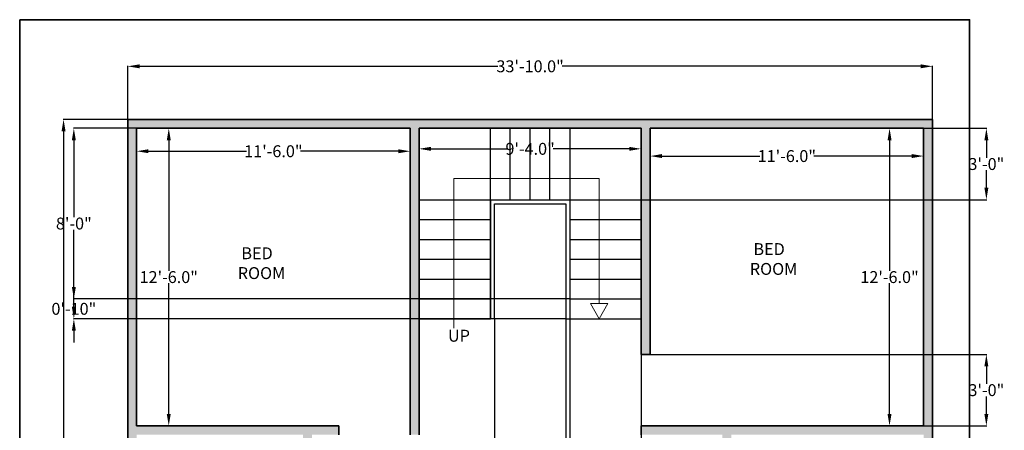
# Model space of a CAD drawing. Units: inches. Extents: x 290 to 786, y 704 to 1301.
# Tile 2 of 2: x 290 to 786, y 1094 to 1301. Entities that reach past the tile are written whole.
import ezdxf

# ---------------------------------------------------------------- set-up
doc = ezdxf.new("R2010")
doc.units = ezdxf.units.IN
doc.header["$MEASUREMENT"] = 0
for name, color, linetype, lineweight in [('A-ANNO-DIMS', 2, 'Continuous', 18), ('A-ANNO-SYMB', 7, 'Continuous', 18), ('A-ANNO-TEXT', 7, 'Continuous', 18), ('A-ANNO-TTLB', 7, 'Continuous', 35), ('A-AREA-IDEN', 150, 'Continuous', 25), ('A-FLOR-STRS', 7, 'Continuous', 25), ('A-WALL', 7, 'Continuous', 35)]:
    doc.layers.add(name, color=color, linetype=linetype, lineweight=lineweight)
doc.layers.add('A-WALL-PATT', color=2, linetype='Continuous', lineweight=13, true_color=0xf1eb1f)
doc.styles.get("Standard").update_dxf_attribs({"font": 'arial.ttf'})
doc.dimstyles.get("Standard").update_dxf_attribs({"dimtxt": 6, "dimasz": 6, "dimexe": 0.18, "dimexo": 0.0625, "dimgap": 0.09, "dimtad": 0, "dimtih": 1, "dimtoh": 1, "dimdec": 1, "dimzin": 0, "dimdsep": 46, "dimlunit": 3, "dimtxsty": 'Standard', "dimcen": 0.09, "dimadec": 0, "dimazin": 0, "dimtfac": 1, "dimtdec": 1, "dimtofl": 0, "dimtmove": 0, "dimatfit": 3, "dimfxl": 1, "dimtolj": 1, "dimtzin": 0, "dimarcsym": 0})

# ---------------------------------------------------------------- blocks, each defined once
blk = doc.blocks.new('*D1')
at = {"layer": 'A-ANNO-DIMS', "color": 0, "lineweight": -2, "transparency": 16777216}
for p, q in [((348.53, 1245.77), (348.53, 1234.1)), ((486.53, 1245.77), (486.53, 1234.1)), ((354.53, 1234.28), (403.92, 1234.28)), ((480.53, 1234.28), (431.14, 1234.28))]:
    blk.add_line(p, q, dxfattribs=at)
at = {"layer": 'A-ANNO-DIMS', "color": 0, "transparency": 16777216}
for points in [[(354.53, 1235.28), (354.53, 1233.28), (348.53, 1234.28)], [(480.53, 1235.28), (480.53, 1233.28), (486.53, 1234.28)]]:
    blk.add_solid(points, dxfattribs=at)
at = {"layer": 'Defpoints', "color": 0, "transparency": 16777216}
for p in [(348.53, 1245.83), (486.53, 1245.83), (486.53, 1234.28)]:
    blk.add_point(p, dxfattribs=at)
at = {"layer": 'A-ANNO-DIMS', "color": 0, "transparency": 16777216, "insert": (417.53, 1234.28), "char_height": 6, "attachment_point": 5}
blk.add_mtext('\\A1;11\'-6.0"', dxfattribs=at)
blk = doc.blocks.new('*D2')
at = {"layer": 'A-ANNO-DIMS', "color": 0, "lineweight": -2, "transparency": 16777216}
for p, q in [((348.6, 1245.83), (364.93, 1245.83)), ((364.75, 1239.83), (364.75, 1173.98)), ((364.75, 1101.83), (364.75, 1167.68)), ((348.6, 1095.83), (364.93, 1095.83))]:
    blk.add_line(p, q, dxfattribs=at)
at = {"layer": 'A-ANNO-DIMS', "color": 0, "transparency": 16777216}
for points in [[(363.75, 1239.83), (365.75, 1239.83), (364.75, 1245.83)], [(363.75, 1101.83), (365.75, 1101.83), (364.75, 1095.83)]]:
    blk.add_solid(points, dxfattribs=at)
at = {"layer": 'Defpoints', "color": 0, "transparency": 16777216}
for p in [(348.53, 1245.83), (364.75, 1245.83), (348.53, 1095.83)]:
    blk.add_point(p, dxfattribs=at)
at = {"layer": 'A-ANNO-DIMS', "color": 0, "transparency": 16777216, "insert": (364.75, 1170.83), "char_height": 6, "attachment_point": 5}
blk.add_mtext('\\A1;12\'-6.0"', dxfattribs=at)
blk = doc.blocks.new('*D3')
at = {"layer": 'A-ANNO-DIMS', "color": 0, "lineweight": -2, "transparency": 16777216}
for p, q in [((491.03, 1245.77), (491.03, 1235.31)), ((603.03, 1245.77), (603.03, 1235.31)), ((497.03, 1235.49), (535.47, 1235.49)), ((597.03, 1235.49), (558.59, 1235.49))]:
    blk.add_line(p, q, dxfattribs=at)
at = {"layer": 'A-ANNO-DIMS', "color": 0, "transparency": 16777216}
for points in [[(497.03, 1236.49), (497.03, 1234.49), (491.03, 1235.49)], [(597.03, 1236.49), (597.03, 1234.49), (603.03, 1235.49)]]:
    blk.add_solid(points, dxfattribs=at)
at = {"layer": 'Defpoints', "color": 0, "transparency": 16777216}
for p in [(491.03, 1245.83), (603.03, 1245.83), (603.03, 1235.49)]:
    blk.add_point(p, dxfattribs=at)
at = {"layer": 'A-ANNO-DIMS', "color": 0, "transparency": 16777216, "insert": (547.03, 1235.49), "char_height": 6, "attachment_point": 5}
blk.add_mtext('\\A1;9\'-4.0"', dxfattribs=at)
blk = doc.blocks.new('*D4')
at = {"layer": 'A-ANNO-DIMS', "color": 0, "lineweight": -2, "transparency": 16777216}
for p, q in [((607.53, 1245.77), (607.53, 1231.66)), ((745.53, 1245.77), (745.53, 1231.66)), ((613.53, 1231.84), (662.92, 1231.84)), ((739.53, 1231.84), (690.14, 1231.84))]:
    blk.add_line(p, q, dxfattribs=at)
at = {"layer": 'A-ANNO-DIMS', "color": 0, "transparency": 16777216}
for points in [[(613.53, 1232.84), (613.53, 1230.84), (607.53, 1231.84)], [(739.53, 1232.84), (739.53, 1230.84), (745.53, 1231.84)]]:
    blk.add_solid(points, dxfattribs=at)
at = {"layer": 'Defpoints', "color": 0, "transparency": 16777216}
for p in [(607.53, 1245.83), (745.53, 1245.83), (745.53, 1231.84)]:
    blk.add_point(p, dxfattribs=at)
at = {"layer": 'A-ANNO-DIMS', "color": 0, "transparency": 16777216, "insert": (676.53, 1231.84), "char_height": 6, "attachment_point": 5}
blk.add_mtext('\\A1;11\'-6.0"', dxfattribs=at)
blk = doc.blocks.new('*D5')
at = {"layer": 'A-ANNO-DIMS', "color": 0, "lineweight": -2, "transparency": 16777216}
for p, q in [((745.47, 1245.83), (728.15, 1245.83)), ((728.33, 1239.83), (728.33, 1173.98)), ((728.33, 1101.83), (728.33, 1167.68)), ((745.47, 1095.83), (728.15, 1095.83))]:
    blk.add_line(p, q, dxfattribs=at)
at = {"layer": 'A-ANNO-DIMS', "color": 0, "transparency": 16777216}
for points in [[(727.33, 1239.83), (729.33, 1239.83), (728.33, 1245.83)], [(727.33, 1101.83), (729.33, 1101.83), (728.33, 1095.83)]]:
    blk.add_solid(points, dxfattribs=at)
at = {"layer": 'Defpoints', "color": 0, "transparency": 16777216}
for p in [(745.53, 1245.83), (728.33, 1095.83), (745.53, 1095.83)]:
    blk.add_point(p, dxfattribs=at)
at = {"layer": 'A-ANNO-DIMS', "color": 0, "transparency": 16777216, "insert": (728.33, 1170.83), "char_height": 6, "attachment_point": 5}
blk.add_mtext('\\A1;12\'-6.0"', dxfattribs=at)
blk = doc.blocks.new('*D17')
at = {"layer": 'A-ANNO-DIMS', "color": 0, "lineweight": -2, "transparency": 16777216}
for p, q in [((344.03, 1250.39), (344.03, 1277.28)), ((350.03, 1277.1), (530.81, 1277.1)), ((744.03, 1277.1), (563.25, 1277.1)), ((750.03, 1250.39), (750.03, 1277.28))]:
    blk.add_line(p, q, dxfattribs=at)
at = {"layer": 'A-ANNO-DIMS', "color": 0, "transparency": 16777216}
for points in [[(350.03, 1278.1), (350.03, 1276.1), (344.03, 1277.1)], [(744.03, 1278.1), (744.03, 1276.1), (750.03, 1277.1)]]:
    blk.add_solid(points, dxfattribs=at)
at = {"layer": 'Defpoints', "color": 0, "transparency": 16777216}
for p in [(750.03, 1277.1), (344.03, 1250.33), (750.03, 1250.33)]:
    blk.add_point(p, dxfattribs=at)
at = {"layer": 'A-ANNO-DIMS', "color": 0, "transparency": 16777216, "insert": (547.03, 1277.1), "char_height": 6, "attachment_point": 5}
blk.add_mtext('\\A1;33\'-10.0"', dxfattribs=at)
blk = doc.blocks.new('*D18')
at = {"layer": 'A-ANNO-DIMS', "color": 0, "lineweight": -2, "transparency": 16777216}
for p, q in [((343.97, 1250.33), (311.5, 1250.33)), ((311.68, 1244.33), (311.68, 1026.48)), ((311.68, 802.33), (311.68, 1020.17)), ((343.97, 796.33), (311.5, 796.33))]:
    blk.add_line(p, q, dxfattribs=at)
at = {"layer": 'A-ANNO-DIMS', "color": 0, "transparency": 16777216}
for points in [[(310.68, 1244.33), (312.68, 1244.33), (311.68, 1250.33)], [(310.68, 802.33), (312.68, 802.33), (311.68, 796.33)]]:
    blk.add_solid(points, dxfattribs=at)
at = {"layer": 'Defpoints', "color": 0, "transparency": 16777216}
for p in [(344.03, 1250.33), (311.68, 796.33), (344.03, 796.33)]:
    blk.add_point(p, dxfattribs=at)
at = {"layer": 'A-ANNO-DIMS', "color": 0, "transparency": 16777216, "insert": (311.68, 1023.33), "char_height": 6, "attachment_point": 5}
blk.add_mtext('\\A1;37\'-10.0"', dxfattribs=at)
blk = doc.blocks.new('*D21')
at = {"layer": 'A-ANNO-DIMS', "color": 0, "lineweight": -2, "transparency": 16777216}
for p, q in [((486.47, 1245.83), (316.7, 1245.83)), ((316.88, 1239.83), (316.88, 1200.98)), ((316.88, 1155.83), (316.88, 1194.68)), ((490.97, 1149.83), (316.7, 1149.83))]:
    blk.add_line(p, q, dxfattribs=at)
at = {"layer": 'A-ANNO-DIMS', "color": 0, "transparency": 16777216}
for points in [[(315.88, 1239.83), (317.88, 1239.83), (316.88, 1245.83)], [(315.88, 1155.83), (317.88, 1155.83), (316.88, 1149.83)]]:
    blk.add_solid(points, dxfattribs=at)
at = {"layer": 'Defpoints', "color": 0, "transparency": 16777216}
for p in [(486.53, 1245.83), (316.88, 1149.83), (491.03, 1149.83)]:
    blk.add_point(p, dxfattribs=at)
at = {"layer": 'A-ANNO-DIMS', "color": 0, "transparency": 16777216, "insert": (316.88, 1197.83), "char_height": 6, "attachment_point": 5}
blk.add_mtext('\\A1;8\'-0"', dxfattribs=at)
blk = doc.blocks.new('*D22')
at = {"layer": 'A-ANNO-DIMS', "color": 0, "lineweight": -2, "transparency": 16777216}
for p, q in [((567.03, 1149.77), (567.03, 712.58)), ((603.03, 1149.77), (603.03, 712.58)), ((573.03, 712.76), (576.97, 712.76)), ((597.03, 712.76), (593.1, 712.76))]:
    blk.add_line(p, q, dxfattribs=at)
at = {"layer": 'A-ANNO-DIMS', "color": 0, "transparency": 16777216}
for points in [[(573.03, 713.76), (573.03, 711.76), (567.03, 712.76)], [(597.03, 713.76), (597.03, 711.76), (603.03, 712.76)]]:
    blk.add_solid(points, dxfattribs=at)
at = {"layer": 'Defpoints', "color": 0, "transparency": 16777216}
for p in [(567.03, 1149.83), (603.03, 1149.83), (603.03, 712.76)]:
    blk.add_point(p, dxfattribs=at)
at = {"layer": 'A-ANNO-DIMS', "color": 0, "transparency": 16777216, "insert": (585.03, 712.76), "char_height": 6, "attachment_point": 5}
blk.add_mtext('\\A1;3\'-0"', dxfattribs=at)
blk = doc.blocks.new('*D23')
at = {"layer": 'A-ANNO-DIMS', "color": 0, "lineweight": -2, "transparency": 16777216}
for p, q in [((316.883325, 1165.829001), (316.883325, 1171.829001)), ((566.970825, 1159.829001), (316.703325, 1159.829001)), ((564.970825, 1149.829001), (316.703325, 1149.829001)), ((316.883325, 1143.829001), (316.883325, 1137.829001))]:
    blk.add_line(p, q, dxfattribs=at)
at = {"layer": 'A-ANNO-DIMS', "color": 0, "transparency": 16777216}
for points in [[(315.883325, 1165.829001), (317.883325, 1165.829001), (316.883325, 1159.829001)], [(315.883325, 1143.829001), (317.883325, 1143.829001), (316.883325, 1149.829001)]]:
    blk.add_solid(points, dxfattribs=at)
at = {"layer": 'Defpoints', "color": 0, "transparency": 16777216}
for p in [(567.033325, 1159.829001), (316.883325, 1149.829001), (565.033325, 1149.829001)]:
    blk.add_point(p, dxfattribs=at)
at = {"layer": 'A-ANNO-DIMS', "color": 0, "transparency": 16777216, "insert": (316.883325, 1154.829001), "char_height": 6, "attachment_point": 5}
blk.add_mtext('\\A1;0\'-10"', dxfattribs=at)
blk = doc.blocks.new('*D24')
at = {"layer": 'A-ANNO-DIMS', "color": 0, "lineweight": -2, "transparency": 16777216}
for p, q in [((529.03, 1149.77), (529.03, 712.58)), ((565.03, 1149.77), (565.03, 712.58)), ((535.03, 712.76), (538.97, 712.76)), ((559.03, 712.76), (555.1, 712.76))]:
    blk.add_line(p, q, dxfattribs=at)
at = {"layer": 'A-ANNO-DIMS', "color": 0, "transparency": 16777216}
for points in [[(535.03, 713.76), (535.03, 711.76), (529.03, 712.76)], [(559.03, 713.76), (559.03, 711.76), (565.03, 712.76)]]:
    blk.add_solid(points, dxfattribs=at)
at = {"layer": 'Defpoints', "color": 0, "transparency": 16777216}
for p in [(529.03, 1149.83), (565.03, 1149.83), (565.03, 712.76)]:
    blk.add_point(p, dxfattribs=at)
at = {"layer": 'A-ANNO-DIMS', "color": 0, "transparency": 16777216, "insert": (547.03, 712.76), "char_height": 6, "attachment_point": 5}
blk.add_mtext('\\A1;3\'-0"', dxfattribs=at)
blk = doc.blocks.new('*D25')
at = {"layer": 'A-ANNO-DIMS', "color": 0, "lineweight": -2, "transparency": 16777216}
for p, q in [((607.6, 1245.83), (777.36, 1245.83)), ((777.18, 1239.83), (777.18, 1230.98)), ((777.18, 1215.83), (777.18, 1224.67)), ((603.1, 1209.83), (777.36, 1209.83))]:
    blk.add_line(p, q, dxfattribs=at)
at = {"layer": 'A-ANNO-DIMS', "color": 0, "transparency": 16777216}
for points in [[(776.18, 1239.83), (778.18, 1239.83), (777.18, 1245.83)], [(776.18, 1215.83), (778.18, 1215.83), (777.18, 1209.83)]]:
    blk.add_solid(points, dxfattribs=at)
at = {"layer": 'Defpoints', "color": 0, "transparency": 16777216}
for p in [(607.53, 1245.83), (777.18, 1245.83), (603.03, 1209.83)]:
    blk.add_point(p, dxfattribs=at)
at = {"layer": 'A-ANNO-DIMS', "color": 0, "transparency": 16777216, "insert": (777.18, 1227.83), "char_height": 6, "attachment_point": 5}
blk.add_mtext('\\A1;3\'-0"', dxfattribs=at)
blk = doc.blocks.new('*D34')
at = {"layer": 'A-ANNO-DIMS', "color": 0, "lineweight": -2, "transparency": 16777216}
for p, q in [((607.6, 1131.83), (777.36, 1131.83)), ((777.18, 1125.83), (777.18, 1116.98)), ((777.18, 1101.83), (777.18, 1110.67)), ((603.1, 1095.83), (777.36, 1095.83))]:
    blk.add_line(p, q, dxfattribs=at)
at = {"layer": 'A-ANNO-DIMS', "color": 0, "transparency": 16777216}
for points in [[(776.18, 1125.83), (778.18, 1125.83), (777.18, 1131.83)], [(776.18, 1101.83), (778.18, 1101.83), (777.18, 1095.83)]]:
    blk.add_solid(points, dxfattribs=at)
at = {"layer": 'Defpoints', "color": 0, "transparency": 16777216}
for p in [(607.53, 1131.83), (777.18, 1131.83), (603.03, 1095.83)]:
    blk.add_point(p, dxfattribs=at)
at = {"layer": 'A-ANNO-DIMS', "color": 0, "transparency": 16777216, "insert": (777.18, 1113.83), "char_height": 6, "attachment_point": 5}
blk.add_mtext('\\A1;3\'-0"', dxfattribs=at)

msp = doc.modelspace()

# ---------------------------------------------------------------- hatches: boundary and pattern name
at = {"layer": 'A-WALL-PATT'}
h = msp.add_hatch(color=256, dxfattribs=at)
h.dxf.hatch_style = 1
h.paths.add_polyline_path([(750.03, 1250.33), (344.03, 1250.33), (344.03, 796.33), (491.03, 796.33), (491.03, 865.83), (567.03, 865.83), (567.03, 870.33), (491.03, 870.33), (491.03, 963.33), (486.53, 963.33), (486.53, 800.83), (348.53, 800.83), (348.53, 958.83), (400.53, 958.83), (400.53, 963.33), (348.53, 963.33), (348.53, 1023.33), (432.53, 1023.33), (432.53, 958.83), (450.53, 958.83), (450.53, 963.33), (437.03, 963.33), (437.03, 1027.83), (348.53, 1027.83), (348.53, 1091.33), (432.53, 1091.33), (432.53, 1059.83), (437.03, 1059.83), (437.03, 1091.33), (450.53, 1091.33), (450.53, 1095.83), (348.53, 1095.83), (348.53, 1245.83), (486.53, 1245.83), (486.53, 1091.33), (491.03, 1091.33), (491.03, 1245.83), (603.03, 1245.83), (603.03, 1131.83), (607.53, 1131.83), (607.53, 1245.83), (745.53, 1245.83), (745.53, 1095.83), (603.03, 1095.83), (603.03, 1091.33), (644.03, 1091.33), (644.03, 1067.33), (648.53, 1067.33), (648.53, 1091.33), (745.53, 1091.33), (745.53, 963.33), (648.53, 963.33), (648.53, 987.33), (644.03, 987.33), (644.03, 963.33), (603.03, 963.33), (603.03, 958.83), (745.53, 958.83), (745.53, 800.83), (607.53, 800.83), (607.53, 922.83), (603.03, 922.83), (603.03, 796.33), (750.03, 796.33)])

# ---------------------------------------------------------------- linework, layer by layer
at = {"layer": 'A-ANNO-SYMB'}
for p, q in [((508.59, 1145.07), (508.59, 1220.55)), ((508.59, 1220.55), (581.83, 1220.55)), ((581.83, 1220.55), (581.83, 1157.49)), ((581.83, 1149.83), (577.42, 1157.49)), ((577.42, 1157.49), (586.24, 1157.49)), ((581.83, 1149.83), (586.24, 1157.49))]:
    msp.add_line(p, q, dxfattribs=at)
at = {"layer": 'A-ANNO-TTLB'}
msp.add_lwpolyline([(289.56, 1300.6), (768.7, 1300.6), (768.7, 731.29), (289.56, 731.29)], close=True, dxfattribs=at)
at = {"layer": 'A-FLOR-STRS'}
for p, q in [((491.03, 1245.83), (491.03, 1209.83)), ((527.03, 1149.83), (527.03, 1245.83)), ((537.03, 1209.83), (537.03, 1245.83)), ((547.03, 1209.83), (547.03, 1245.83)), ((557.03, 1209.83), (557.03, 1245.83)), ((603.03, 1245.83), (567.03, 1245.83)), ((567.03, 1245.83), (567.03, 1149.83)), ((491.03, 1209.83), (603.03, 1209.83)), ((491.03, 1209.83), (527.03, 1209.83)), ((527.03, 1209.83), (527.03, 1149.83)), ((529.03, 1149.83), (529.03, 1207.83)), ((529.03, 1207.83), (565.03, 1207.83)), ((565.03, 1207.83), (565.03, 1149.83)), ((491.03, 1199.83), (527.03, 1199.83)), ((491.03, 1199.83), (527.03, 1199.83)), ((567.03, 1199.83), (603.03, 1199.83)), ((491.03, 1189.83), (527.03, 1189.83)), ((491.03, 1189.83), (527.03, 1189.83)), ((567.03, 1189.83), (603.03, 1189.83)), ((491.03, 1179.83), (527.03, 1179.83)), ((491.03, 1179.83), (527.03, 1179.83)), ((567.03, 1179.83), (603.03, 1179.83)), ((491.03, 1169.83), (527.03, 1169.83)), ((491.03, 1169.83), (527.03, 1169.83)), ((567.03, 1169.83), (603.03, 1169.83)), ((491.03, 1159.83), (527.03, 1159.83)), ((491.03, 1159.83), (527.03, 1159.83)), ((567.03, 1159.83), (603.03, 1159.83)), ((491.03, 1149.83), (527.03, 1149.83)), ((491.03, 1149.83), (527.03, 1149.83)), ((529.03, 1149.83), (527.03, 1149.83)), ((565.03, 1149.83), (567.03, 1149.83)), ((567.03, 1149.83), (603.03, 1149.83))]:
    msp.add_line(p, q, dxfattribs=at)
at = {"layer": 'A-WALL'}
for p, q in [((344.03, 1250.33), (750.03, 1250.33)), ((344.03, 1250.33), (344.03, 796.33)), ((750.03, 1250.33), (750.03, 796.33)), ((348.53, 1245.83), (348.53, 1095.83)), ((348.53, 1245.83), (486.53, 1245.83)), ((486.53, 1245.83), (486.53, 1091.33)), ((491.03, 1245.83), (491.03, 1091.33)), ((491.03, 1245.83), (603.03, 1245.83)), ((603.03, 1245.83), (603.03, 1131.83)), ((607.53, 1245.83), (607.53, 1131.83)), ((607.53, 1245.83), (745.53, 1245.83)), ((745.53, 1245.83), (745.53, 1095.83)), ((603.03, 1131.83), (607.53, 1131.83)), ((348.53, 1095.83), (450.53, 1095.83)), ((450.53, 1091.33), (450.53, 1095.83)), ((603.03, 1095.83), (745.53, 1095.83)), ((603.03, 1095.83), (603.03, 1091.33))]:
    msp.add_line(p, q, dxfattribs=at)

# ---------------------------------------------------------------- texts
at = {"layer": 'A-ANNO-TEXT', "insert": (505.6, 1144.26), "char_height": 6, "attachment_point": 1}
msp.add_mtext_dynamic_manual_height_columns('UP', width=8.7965, gutter_width=30, heights=[0], dxfattribs=at)
at = {"layer": 'A-AREA-IDEN', "char_height": 6, "attachment_point": 1}
for width, insert in [(37.6486, (657.84, 1187.94)), (43.6889, (399.54, 1185.84))]:
    msp.add_mtext_dynamic_manual_height_columns(' BED\\PROOM', width=width, gutter_width=30, heights=[0], dxfattribs=dict(at, insert=insert))

# ---------------------------------------------------------------- dimensions: what is measured, and where the dimension line sits
at = {"layer": 'A-ANNO-DIMS'}
for base, p1, p2, override, picture, middle in [((750.03, 1277.1), (344.03, 1250.33), (750.03, 1250.33), {"dimclrd": 0, "dimclre": 0, "dimclrt": 0}, '*D17', (547.03, 1277.1)), ((486.53, 1234.28), (348.53, 1245.83), (486.53, 1245.83), {"dimclrd": 0, "dimclre": 0, "dimclrt": 0}, '*D1', (417.53, 1234.28)), ((603.03, 1235.49), (491.03, 1245.83), (603.03, 1245.83), {"dimclrd": 0, "dimclre": 0, "dimclrt": 0}, '*D3', (547.03, 1235.49)), ((745.53, 1231.84), (607.53, 1245.83), (745.53, 1245.83), {"dimclrd": 0, "dimclre": 0, "dimclrt": 0}, '*D4', (676.53, 1231.84)), ((565.03, 712.76), (529.03, 1149.83), (565.03, 1149.83), {"dimdec": 1, "dimlfac": 1, "dimrnd": 0, "dimzin": 1, "dimdsep": 46, "dimlunit": 4, "dimfrac": 2}, '*D24', (547.03, 712.76)), ((603.03, 712.76), (567.03, 1149.83), (603.03, 1149.83), {"dimdec": 1, "dimlfac": 1, "dimrnd": 0, "dimzin": 1, "dimdsep": 46, "dimlunit": 4, "dimfrac": 2}, '*D22', (585.03, 712.76))]:
    dim = msp.add_linear_dim(base=base, p1=p1, p2=p2, dimstyle='Standard', override=override, dxfattribs=at)
    dim.commit()
    dim.dimension.update_dxf_attribs({"geometry": picture, "text_midpoint": middle})
for base, p1, p2, override, picture, middle in [((311.68, 796.33), (344.03, 1250.33), (344.03, 796.33), {"dimclrd": 0, "dimclre": 0, "dimclrt": 0}, '*D18', (311.68, 1023.33)), ((316.88, 1149.83), (486.53, 1245.83), (491.03, 1149.83), {"dimdec": 1, "dimlfac": 1, "dimrnd": 0, "dimzin": 1, "dimdsep": 46, "dimlunit": 4, "dimfrac": 2}, '*D21', (316.88, 1197.83)), ((364.75, 1245.83), (348.53, 1095.83), (348.53, 1245.83), {"dimclrd": 0, "dimclre": 0, "dimclrt": 0}, '*D2', (364.75, 1170.83)), ((777.18, 1245.83), (603.03, 1209.83), (607.53, 1245.83), {"dimdec": 1, "dimlfac": 1, "dimrnd": 0, "dimzin": 1, "dimdsep": 46, "dimlunit": 4, "dimfrac": 2}, '*D25', (777.18, 1227.83)), ((728.33, 1095.83), (745.53, 1245.83), (745.53, 1095.83), {"dimclrd": 0, "dimclre": 0, "dimclrt": 0}, '*D5', (728.33, 1170.83)), ((316.88, 1149.83), (567.03, 1159.83), (565.03, 1149.83), {"dimdec": 1, "dimlfac": 1, "dimrnd": 0, "dimzin": 1, "dimdsep": 46, "dimlunit": 4, "dimfrac": 2}, '*D23', (316.88, 1154.83)), ((777.18, 1131.83), (603.03, 1095.83), (607.53, 1131.83), {"dimdec": 1, "dimlfac": 1, "dimrnd": 0, "dimzin": 1, "dimdsep": 46, "dimlunit": 4, "dimfrac": 2}, '*D34', (777.18, 1113.83))]:
    dim = msp.add_linear_dim(base=base, p1=p1, p2=p2, angle=90, dimstyle='Standard', override=override, dxfattribs=at)
    dim.commit()
    dim.dimension.update_dxf_attribs({"geometry": picture, "text_midpoint": middle})

doc.saveas('drawing.dxf')
